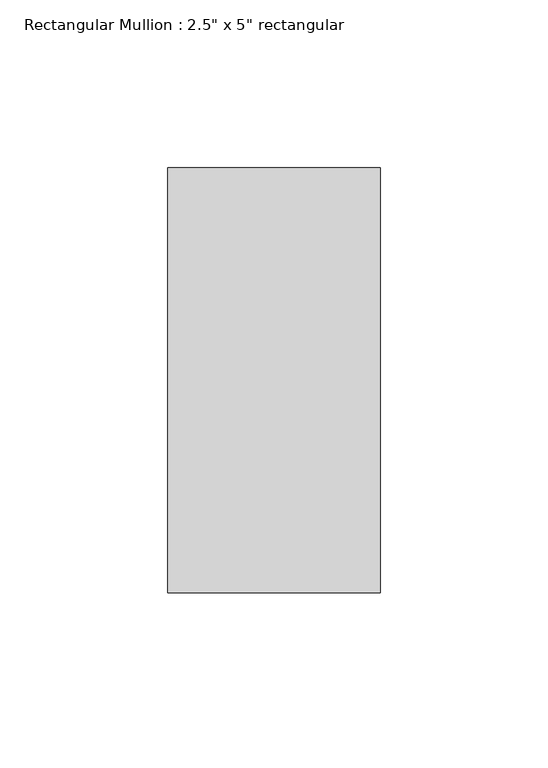
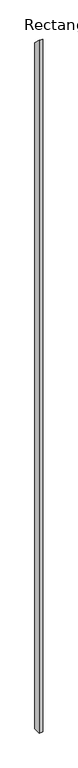
"""IFC4 building model written with IfcOpenShell, lengths in millimetres: member geometry."""

from ifc_helpers import new_model, si_unit, frame, origin, place, context, project, spatial, polyline, outline, extrude, source, transform, mapped, element, save


def member_19d8ec5e(model_context):
    return source(origin(), model_context, "Body", "SweptSolid", [
        extrude(outline(polyline([(-63.5, 63.5), (63.5, -63.5), (63.5, -12758.7552746), (-63.5, -12758.7552746), (-63.5, 63.5)])), frame((-63.5, 0.0, 0.0), z_axis=(1.0, 0.0, 0.0), x_axis=(0.0, 1.0, 0.0)), (0.0, 0.0, 1.0), 63.5),
    ])


if __name__ == "__main__":
    model = new_model("IFC4")
    model_context = context("Model", 3, world=origin())
    ifc_project = project(units=[si_unit("LENGTHUNIT", "METRE", prefix="MILLI")], contexts=[model_context])
    site = spatial("IfcSite", under=ifc_project)
    building = spatial("IfcBuilding", under=site)
    placement = place(None, origin())
    member_shape = member_19d8ec5e(model_context)
    element("IfcMember", 1, ObjectType="Rectangular Mullion : 2.5\" x 5\" rectangular", at=placement, inside=building, context=model_context, shape_type="MappedRepresentation", body=[
        mapped(member_shape, transform((0.0, 0.0, 0.0), x_axis=(1.0, 0.0, 0.0), y_axis=(0.0, 1.0, 0.0), z_axis=(0.0, 0.0, 1.0))),
    ])
    save(model, "model.ifc")

# Revit data of these elements
# Type "Rectangular Mullion : 2.5\" x 5\" rectangular"
#   built-in parameter 1007304 = 0.416667 (stored number, unit not read)
#   built-in parameter 1007301 = 0.104167 (stored number, unit not read)
#   built-in parameter 1007300 = 0.104167 (stored number, unit not read)
# Element 1 (IfcMember, "Rectangular Mullion : 2.5\" x 5\" rectangular")
#   Materials on its faces: "Aluminum"
# Materials
#   "Aluminum": class "Metal", colour RGB 247 247 247, transparency 0, Description = "Aluminum 6061", Cost = 0
